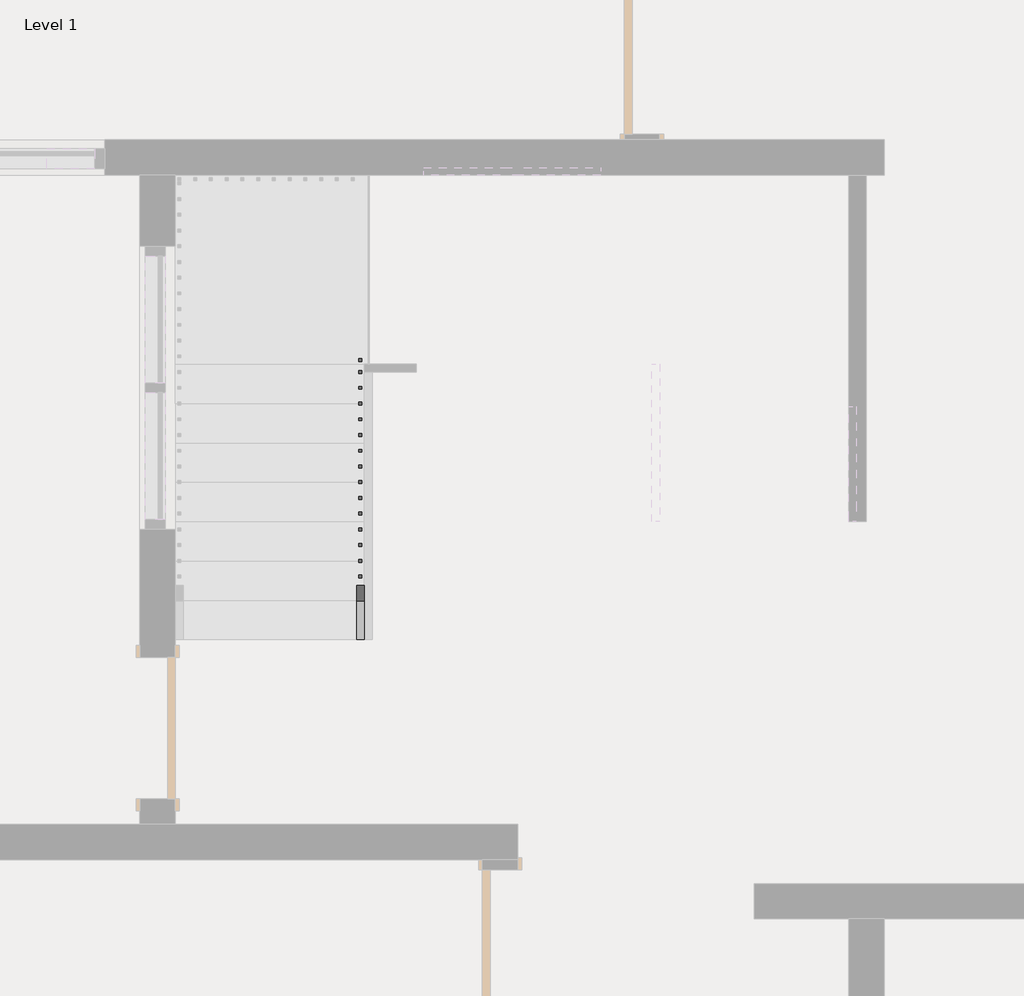
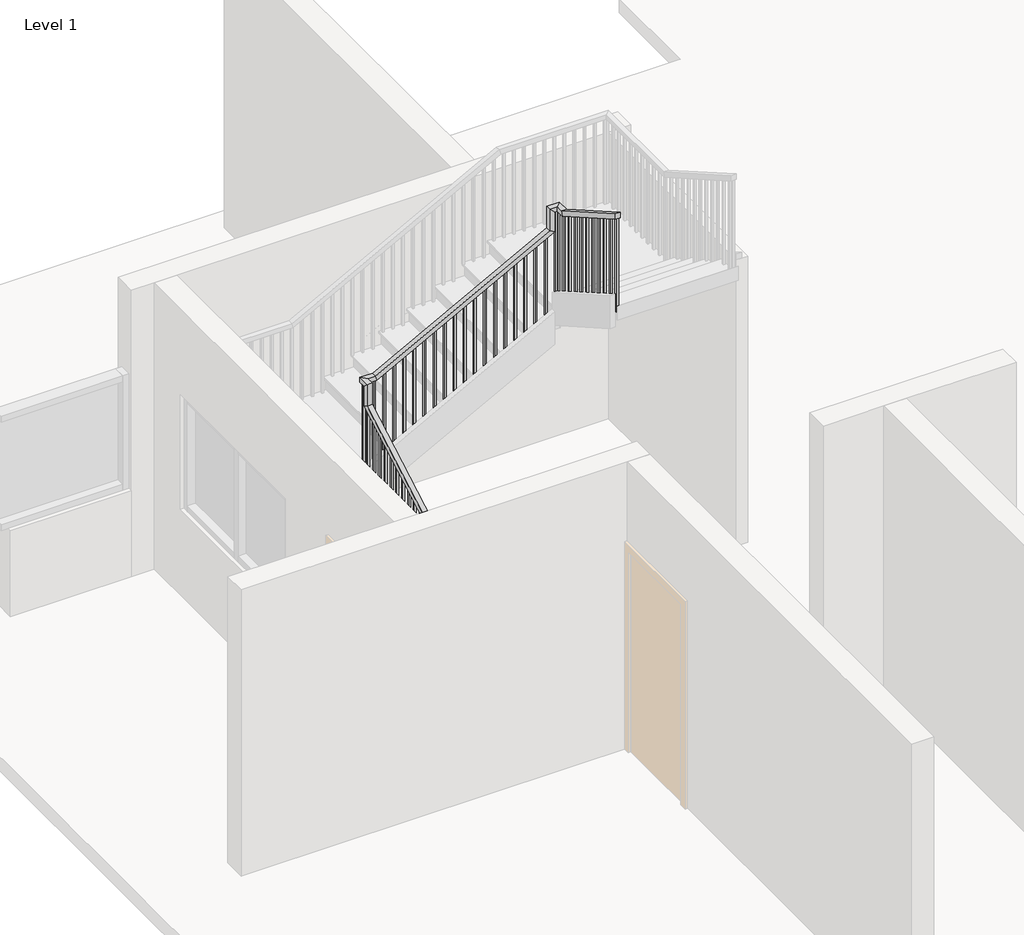
# One storey, part 8 of 9: 1 railing.
"""IFC4 building model written with IfcOpenShell, lengths in millimetres."""

from ifc_helpers import new_model, si_unit, frame, origin, place, context, project, spatial, polyline, outline, extrude, faceted_brep, element, save

model = new_model("IFC4")

# Units and contexts
model_context = context("Model", 3, world=origin())
ifc_project = project(units=[si_unit("LENGTHUNIT", "METRE", prefix="MILLI")], contexts=[model_context])

# Site, building, storey
site = spatial("IfcSite", under=ifc_project)
building = spatial("IfcBuilding", under=site)
storey = spatial("IfcBuildingStorey", under=building, Name="Level 1", Elevation=0.0)

# Railing
placement = place(None, origin())
element("IfcRailing", 1, ObjectType="Handrail - Rectangular", at=placement, inside=storey, context=model_context, shape_type="SolidModel", body=[
    faceted_brep([(14461.3100959, 14647.8480703, 1059.5428571), (14461.3100959, 14647.8480703, 1001.0339009), (14512.1100959, 14647.8480703, 1001.0339009), (14512.1100959, 14647.8480703, 1059.5428571), (14461.3100959, 16349.6480703, 2032.0), (14461.3100959, 16400.4480703, 2002.5196152), (14512.1100959, 16400.4480703, 2002.5196152), (14512.1100959, 16349.6480703, 2032.0), (14461.3100959, 16349.6480703, 2261.3257143), (14461.3100959, 16400.4480703, 2210.5257143), (14512.1100959, 16400.4480703, 2210.5257143), (14512.1100959, 16349.6480703, 2261.3257143), (14461.3100959, 16476.6480703, 2261.3257143), (14461.3100959, 16476.6480703, 2210.5257143), (14512.1100959, 16425.8480703, 2210.5257143), (14512.1100959, 16425.8480703, 2261.3257143), (14588.3100959, 16476.6480703, 2261.3257143), (14601.0100959, 16476.6480703, 2210.5257143), (14601.0100959, 16425.8480703, 2210.5257143), (14588.3100959, 16425.8480703, 2261.3257143), (16340.9100959, 16476.6480703, 3196.0457143), (16391.7100959, 16476.6480703, 3165.5657143), (16391.7100959, 16425.8480703, 3165.5657143), (16340.9100959, 16425.8480703, 3196.0457143), (16340.9100959, 16476.6480703, 3425.3714286), (16391.7100959, 16476.6480703, 3374.5714286), (16391.7100959, 16425.8480703, 3374.5714286), (16340.9100959, 16425.8480703, 3425.3714286), (16467.9100959, 16476.6480703, 3425.3714286), (16467.9100959, 16476.6480703, 3374.5714286), (16417.1100959, 16425.8480703, 3374.5714286), (16417.1100959, 16425.8480703, 3425.3714286), (16467.9100959, 16349.6480703, 3425.3714286), (16467.9100959, 16336.1573969, 3374.5714286), (16417.1100959, 16336.1573969, 3374.5714286), (16417.1100959, 16349.6480703, 3425.3714286), (16467.9100959, 15409.8480703, 3962.4), (16417.1100959, 15409.8480703, 3962.4), (16417.1100959, 15409.8480703, 3903.8910438), (16467.9100959, 15409.8480703, 3903.8910438)], [[[0, 1, 2, 3]], [[1, 0, 4, 5]], [[2, 1, 5, 6]], [[3, 2, 6, 7]], [[0, 3, 7, 4]], [[5, 4, 8, 9]], [[6, 5, 9, 10]], [[7, 6, 10, 11]], [[4, 7, 11, 8]], [[9, 8, 12, 13]], [[10, 9, 13, 14]], [[11, 10, 14, 15]], [[8, 11, 15, 12]], [[13, 12, 16, 17]], [[14, 13, 17, 18]], [[15, 14, 18, 19]], [[12, 15, 19, 16]], [[17, 16, 20, 21]], [[18, 17, 21, 22]], [[19, 18, 22, 23]], [[16, 19, 23, 20]], [[21, 20, 24, 25]], [[22, 21, 25, 26]], [[23, 22, 26, 27]], [[20, 23, 27, 24]], [[25, 24, 28, 29]], [[26, 25, 29, 30]], [[27, 26, 30, 31]], [[24, 27, 31, 28]], [[29, 28, 32, 33]], [[30, 29, 33, 34]], [[31, 30, 34, 35]], [[28, 31, 35, 32]], [[36, 37, 38, 39]], [[33, 32, 36, 39]], [[34, 33, 39, 38]], [[35, 34, 38, 37]], [[32, 35, 37, 36]]]),
    extrude(outline(polyline([(15425.7230703, 3894.8196152), (15444.7730703, 3883.9339009), (15444.7730703, 2902.8571429), (15425.7230703, 2902.8571429), (15425.7230703, 3894.8196152)])), frame((16432.9850959, 0.0, 0.0), z_axis=(1.0, 0.0, 0.0), x_axis=(0.0, 1.0, 0.0)), (0.0, 0.0, 1.0), 19.05),
    extrude(outline(polyline([(15527.3230703, 3836.7624723), (15546.3730703, 3825.8767581), (15546.3730703, 2902.8571429), (15527.3230703, 2902.8571429), (15527.3230703, 3836.7624723)])), frame((16432.9850959, 0.0, 0.0), z_axis=(1.0, 0.0, 0.0), x_axis=(0.0, 1.0, 0.0)), (0.0, 0.0, 1.0), 19.05),
    extrude(outline(polyline([(15628.9230703, 3778.7053295), (15647.9730703, 3767.8196152), (15647.9730703, 2902.8571429), (15628.9230703, 2902.8571429), (15628.9230703, 3778.7053295)])), frame((16432.9850959, 0.0, 0.0), z_axis=(1.0, 0.0, 0.0), x_axis=(0.0, 1.0, 0.0)), (0.0, 0.0, 1.0), 19.05),
    extrude(outline(polyline([(15730.5230703, 3720.6481866), (15749.5730703, 3709.7624723), (15749.5730703, 2757.7142857), (15730.5230703, 2757.7142857), (15730.5230703, 3720.6481866)])), frame((16432.9850959, 0.0, 0.0), z_axis=(1.0, 0.0, 0.0), x_axis=(0.0, 1.0, 0.0)), (0.0, 0.0, 1.0), 19.05),
    extrude(outline(polyline([(15832.1230703, 3662.5910438), (15851.1730703, 3651.7053295), (15851.1730703, 2757.7142857), (15832.1230703, 2757.7142857), (15832.1230703, 3662.5910438)])), frame((16432.9850959, 0.0, 0.0), z_axis=(1.0, 0.0, 0.0), x_axis=(0.0, 1.0, 0.0)), (0.0, 0.0, 1.0), 19.05),
    extrude(outline(polyline([(15933.7230703, 3604.5339009), (15952.7730703, 3593.6481866), (15952.7730703, 2612.5714286), (15933.7230703, 2612.5714286), (15933.7230703, 3604.5339009)])), frame((16432.9850959, 0.0, 0.0), z_axis=(1.0, 0.0, 0.0), x_axis=(0.0, 1.0, 0.0)), (0.0, 0.0, 1.0), 19.05),
    extrude(outline(polyline([(16035.3230703, 3546.4767581), (16054.3730703, 3535.5910438), (16054.3730703, 2612.5714286), (16035.3230703, 2612.5714286), (16035.3230703, 3546.4767581)])), frame((16432.9850959, 0.0, 0.0), z_axis=(1.0, 0.0, 0.0), x_axis=(0.0, 1.0, 0.0)), (0.0, 0.0, 1.0), 19.05),
    extrude(outline(polyline([(16136.9230703, 3488.4196152), (16155.9730703, 3477.5339009), (16155.9730703, 2612.5714286), (16136.9230703, 2612.5714286), (16136.9230703, 3488.4196152)])), frame((16432.9850959, 0.0, 0.0), z_axis=(1.0, 0.0, 0.0), x_axis=(0.0, 1.0, 0.0)), (0.0, 0.0, 1.0), 19.05),
    extrude(outline(polyline([(16238.5230703, 3430.3624723), (16257.5730703, 3419.4767581), (16257.5730703, 2467.4285714), (16238.5230703, 2467.4285714), (16238.5230703, 3430.3624723)])), frame((16432.9850959, 0.0, 0.0), z_axis=(1.0, 0.0, 0.0), x_axis=(0.0, 1.0, 0.0)), (0.0, 0.0, 1.0), 19.05),
    extrude(outline(polyline([(16340.1230703, 3372.3053295), (16359.1730703, 3361.4196152), (16359.1730703, 2467.4285714), (16340.1230703, 2467.4285714), (16340.1230703, 3372.3053295)])), frame((16432.9850959, 0.0, 0.0), z_axis=(1.0, 0.0, 0.0), x_axis=(0.0, 1.0, 0.0)), (0.0, 0.0, 1.0), 19.05),
    extrude(outline(polyline([(16407.5850959, 16441.7230703), (16407.5850959, 16460.7730703), (16426.6350959, 16460.7730703), (16426.6350959, 16441.7230703), (16407.5850959, 16441.7230703)])), frame((0.0, 0.0, 2322.2857143), z_axis=(0.0, 0.0, 1.0), x_axis=(1.0, 0.0, 0.0)), (0.0, 0.0, 1.0), 1052.2857143),
    extrude(outline(polyline([(3130.0057143, 16325.0350959), (3119.8457143, 16305.9850959), (2177.1428571, 16305.9850959), (2177.1428571, 16325.0350959), (3130.0057143, 16325.0350959)])), frame((0.0, 16441.7230703, 0.0), z_axis=(0.0, 1.0, 0.0), x_axis=(0.0, 0.0, 1.0)), (0.0, 0.0, 1.0), 19.05),
    extrude(outline(polyline([(3075.8190476, 16223.4350959), (3065.6590476, 16204.3850959), (2177.1428571, 16204.3850959), (2177.1428571, 16223.4350959), (3075.8190476, 16223.4350959)])), frame((0.0, 16441.7230703, 0.0), z_axis=(0.0, 1.0, 0.0), x_axis=(0.0, 0.0, 1.0)), (0.0, 0.0, 1.0), 19.05),
    extrude(outline(polyline([(3021.632381, 16121.8350959), (3011.472381, 16102.7850959), (2032.0, 16102.7850959), (2032.0, 16121.8350959), (3021.632381, 16121.8350959)])), frame((0.0, 16441.7230703, 0.0), z_axis=(0.0, 1.0, 0.0), x_axis=(0.0, 0.0, 1.0)), (0.0, 0.0, 1.0), 19.05),
    extrude(outline(polyline([(2967.4457143, 16020.2350959), (2957.2857143, 16001.1850959), (2032.0, 16001.1850959), (2032.0, 16020.2350959), (2967.4457143, 16020.2350959)])), frame((0.0, 16441.7230703, 0.0), z_axis=(0.0, 1.0, 0.0), x_axis=(0.0, 0.0, 1.0)), (0.0, 0.0, 1.0), 19.05),
    extrude(outline(polyline([(2913.2590476, 15918.6350959), (2903.0990476, 15899.5850959), (2032.0, 15899.5850959), (2032.0, 15918.6350959), (2913.2590476, 15918.6350959)])), frame((0.0, 16441.7230703, 0.0), z_axis=(0.0, 1.0, 0.0), x_axis=(0.0, 0.0, 1.0)), (0.0, 0.0, 1.0), 19.05),
    extrude(outline(polyline([(2859.072381, 15817.0350959), (2848.912381, 15797.9850959), (1886.8571429, 15797.9850959), (1886.8571429, 15817.0350959), (2859.072381, 15817.0350959)])), frame((0.0, 16441.7230703, 0.0), z_axis=(0.0, 1.0, 0.0), x_axis=(0.0, 0.0, 1.0)), (0.0, 0.0, 1.0), 19.05),
    extrude(outline(polyline([(2804.8857143, 15715.4350959), (2794.7257143, 15696.3850959), (1886.8571429, 15696.3850959), (1886.8571429, 15715.4350959), (2804.8857143, 15715.4350959)])), frame((0.0, 16441.7230703, 0.0), z_axis=(0.0, 1.0, 0.0), x_axis=(0.0, 0.0, 1.0)), (0.0, 0.0, 1.0), 19.05),
    extrude(outline(polyline([(2750.6990476, 15613.8350959), (2740.5390476, 15594.7850959), (1886.8571429, 15594.7850959), (1886.8571429, 15613.8350959), (2750.6990476, 15613.8350959)])), frame((0.0, 16441.7230703, 0.0), z_axis=(0.0, 1.0, 0.0), x_axis=(0.0, 0.0, 1.0)), (0.0, 0.0, 1.0), 19.05),
    extrude(outline(polyline([(2696.512381, 15512.2350959), (2686.352381, 15493.1850959), (1741.7142857, 15493.1850959), (1741.7142857, 15512.2350959), (2696.512381, 15512.2350959)])), frame((0.0, 16441.7230703, 0.0), z_axis=(0.0, 1.0, 0.0), x_axis=(0.0, 0.0, 1.0)), (0.0, 0.0, 1.0), 19.05),
    extrude(outline(polyline([(2642.3257143, 15410.6350959), (2632.1657143, 15391.5850959), (1741.7142857, 15391.5850959), (1741.7142857, 15410.6350959), (2642.3257143, 15410.6350959)])), frame((0.0, 16441.7230703, 0.0), z_axis=(0.0, 1.0, 0.0), x_axis=(0.0, 0.0, 1.0)), (0.0, 0.0, 1.0), 19.05),
    extrude(outline(polyline([(2588.1390476, 15309.0350959), (2577.9790476, 15289.9850959), (1596.5714286, 15289.9850959), (1596.5714286, 15309.0350959), (2588.1390476, 15309.0350959)])), frame((0.0, 16441.7230703, 0.0), z_axis=(0.0, 1.0, 0.0), x_axis=(0.0, 0.0, 1.0)), (0.0, 0.0, 1.0), 19.05),
    extrude(outline(polyline([(2533.952381, 15207.4350959), (2523.792381, 15188.3850959), (1596.5714286, 15188.3850959), (1596.5714286, 15207.4350959), (2533.952381, 15207.4350959)])), frame((0.0, 16441.7230703, 0.0), z_axis=(0.0, 1.0, 0.0), x_axis=(0.0, 0.0, 1.0)), (0.0, 0.0, 1.0), 19.05),
    extrude(outline(polyline([(2479.7657143, 15105.8350959), (2469.6057143, 15086.7850959), (1596.5714286, 15086.7850959), (1596.5714286, 15105.8350959), (2479.7657143, 15105.8350959)])), frame((0.0, 16441.7230703, 0.0), z_axis=(0.0, 1.0, 0.0), x_axis=(0.0, 0.0, 1.0)), (0.0, 0.0, 1.0), 19.05),
    extrude(outline(polyline([(2425.5790476, 15004.2350959), (2415.4190476, 14985.1850959), (1451.4285714, 14985.1850959), (1451.4285714, 15004.2350959), (2425.5790476, 15004.2350959)])), frame((0.0, 16441.7230703, 0.0), z_axis=(0.0, 1.0, 0.0), x_axis=(0.0, 0.0, 1.0)), (0.0, 0.0, 1.0), 19.05),
    extrude(outline(polyline([(2371.392381, 14902.6350959), (2361.232381, 14883.5850959), (1451.4285714, 14883.5850959), (1451.4285714, 14902.6350959), (2371.392381, 14902.6350959)])), frame((0.0, 16441.7230703, 0.0), z_axis=(0.0, 1.0, 0.0), x_axis=(0.0, 0.0, 1.0)), (0.0, 0.0, 1.0), 19.05),
    extrude(outline(polyline([(2317.2057143, 14801.0350959), (2307.0457143, 14781.9850959), (1451.4285714, 14781.9850959), (1451.4285714, 14801.0350959), (2317.2057143, 14801.0350959)])), frame((0.0, 16441.7230703, 0.0), z_axis=(0.0, 1.0, 0.0), x_axis=(0.0, 0.0, 1.0)), (0.0, 0.0, 1.0), 19.05),
    extrude(outline(polyline([(2263.0190476, 14699.4350959), (2252.8590476, 14680.3850959), (1306.2857143, 14680.3850959), (1306.2857143, 14699.4350959), (2263.0190476, 14699.4350959)])), frame((0.0, 16441.7230703, 0.0), z_axis=(0.0, 1.0, 0.0), x_axis=(0.0, 0.0, 1.0)), (0.0, 0.0, 1.0), 19.05),
    extrude(outline(polyline([(2208.832381, 14597.8350959), (2198.672381, 14578.7850959), (1306.2857143, 14578.7850959), (1306.2857143, 14597.8350959), (2208.832381, 14597.8350959)])), frame((0.0, 16441.7230703, 0.0), z_axis=(0.0, 1.0, 0.0), x_axis=(0.0, 0.0, 1.0)), (0.0, 0.0, 1.0), 19.05),
    extrude(outline(polyline([(14496.2350959, 16365.5230703), (14477.1850959, 16365.5230703), (14477.1850959, 16384.5730703), (14496.2350959, 16384.5730703), (14496.2350959, 16365.5230703)])), frame((0.0, 0.0, 1016.0), z_axis=(0.0, 0.0, 1.0), x_axis=(1.0, 0.0, 0.0)), (0.0, 0.0, 1.0), 1194.5257143),
    extrude(outline(polyline([(16263.9230703, 1924.5053295), (16282.9730703, 1935.3910438), (16282.9730703, 1016.0), (16263.9230703, 1016.0), (16263.9230703, 1924.5053295)])), frame((14477.1850959, 0.0, 0.0), z_axis=(1.0, 0.0, 0.0), x_axis=(0.0, 1.0, 0.0)), (0.0, 0.0, 1.0), 19.05),
    extrude(outline(polyline([(16162.3230703, 1866.4481866), (16181.3730703, 1877.3339009), (16181.3730703, 1016.0), (16162.3230703, 1016.0), (16162.3230703, 1866.4481866)])), frame((14477.1850959, 0.0, 0.0), z_axis=(1.0, 0.0, 0.0), x_axis=(0.0, 1.0, 0.0)), (0.0, 0.0, 1.0), 19.05),
    extrude(outline(polyline([(16060.7230703, 1808.3910438), (16079.7730703, 1819.2767581), (16079.7730703, 870.8571429), (16060.7230703, 870.8571429), (16060.7230703, 1808.3910438)])), frame((14477.1850959, 0.0, 0.0), z_axis=(1.0, 0.0, 0.0), x_axis=(0.0, 1.0, 0.0)), (0.0, 0.0, 1.0), 19.05),
    extrude(outline(polyline([(15959.1230703, 1750.3339009), (15978.1730703, 1761.2196152), (15978.1730703, 870.8571429), (15959.1230703, 870.8571429), (15959.1230703, 1750.3339009)])), frame((14477.1850959, 0.0, 0.0), z_axis=(1.0, 0.0, 0.0), x_axis=(0.0, 1.0, 0.0)), (0.0, 0.0, 1.0), 19.05),
    extrude(outline(polyline([(15857.5230703, 1692.2767581), (15876.5730703, 1703.1624723), (15876.5730703, 725.7142857), (15857.5230703, 725.7142857), (15857.5230703, 1692.2767581)])), frame((14477.1850959, 0.0, 0.0), z_axis=(1.0, 0.0, 0.0), x_axis=(0.0, 1.0, 0.0)), (0.0, 0.0, 1.0), 19.05),
    extrude(outline(polyline([(15755.9230703, 1634.2196152), (15774.9730703, 1645.1053295), (15774.9730703, 725.7142857), (15755.9230703, 725.7142857), (15755.9230703, 1634.2196152)])), frame((14477.1850959, 0.0, 0.0), z_axis=(1.0, 0.0, 0.0), x_axis=(0.0, 1.0, 0.0)), (0.0, 0.0, 1.0), 19.05),
    extrude(outline(polyline([(15654.3230703, 1576.1624723), (15673.3730703, 1587.0481866), (15673.3730703, 725.7142857), (15654.3230703, 725.7142857), (15654.3230703, 1576.1624723)])), frame((14477.1850959, 0.0, 0.0), z_axis=(1.0, 0.0, 0.0), x_axis=(0.0, 1.0, 0.0)), (0.0, 0.0, 1.0), 19.05),
    extrude(outline(polyline([(15552.7230703, 1518.1053295), (15571.7730703, 1528.9910438), (15571.7730703, 580.5714286), (15552.7230703, 580.5714286), (15552.7230703, 1518.1053295)])), frame((14477.1850959, 0.0, 0.0), z_axis=(1.0, 0.0, 0.0), x_axis=(0.0, 1.0, 0.0)), (0.0, 0.0, 1.0), 19.05),
    extrude(outline(polyline([(15451.1230703, 1460.0481866), (15470.1730703, 1470.9339009), (15470.1730703, 580.5714286), (15451.1230703, 580.5714286), (15451.1230703, 1460.0481866)])), frame((14477.1850959, 0.0, 0.0), z_axis=(1.0, 0.0, 0.0), x_axis=(0.0, 1.0, 0.0)), (0.0, 0.0, 1.0), 19.05),
    extrude(outline(polyline([(15349.5230703, 1401.9910438), (15368.5730703, 1412.8767581), (15368.5730703, 435.4285714), (15349.5230703, 435.4285714), (15349.5230703, 1401.9910438)])), frame((14477.1850959, 0.0, 0.0), z_axis=(1.0, 0.0, 0.0), x_axis=(0.0, 1.0, 0.0)), (0.0, 0.0, 1.0), 19.05),
    extrude(outline(polyline([(15247.9230703, 1343.9339009), (15266.9730703, 1354.8196152), (15266.9730703, 435.4285714), (15247.9230703, 435.4285714), (15247.9230703, 1343.9339009)])), frame((14477.1850959, 0.0, 0.0), z_axis=(1.0, 0.0, 0.0), x_axis=(0.0, 1.0, 0.0)), (0.0, 0.0, 1.0), 19.05),
    extrude(outline(polyline([(15146.3230703, 1285.8767581), (15165.3730703, 1296.7624723), (15165.3730703, 435.4285714), (15146.3230703, 435.4285714), (15146.3230703, 1285.8767581)])), frame((14477.1850959, 0.0, 0.0), z_axis=(1.0, 0.0, 0.0), x_axis=(0.0, 1.0, 0.0)), (0.0, 0.0, 1.0), 19.05),
    extrude(outline(polyline([(15044.7230703, 1227.8196152), (15063.7730703, 1238.7053295), (15063.7730703, 290.2857143), (15044.7230703, 290.2857143), (15044.7230703, 1227.8196152)])), frame((14477.1850959, 0.0, 0.0), z_axis=(1.0, 0.0, 0.0), x_axis=(0.0, 1.0, 0.0)), (0.0, 0.0, 1.0), 19.05),
    extrude(outline(polyline([(14943.1230703, 1169.7624723), (14962.1730703, 1180.6481866), (14962.1730703, 290.2857143), (14943.1230703, 290.2857143), (14943.1230703, 1169.7624723)])), frame((14477.1850959, 0.0, 0.0), z_axis=(1.0, 0.0, 0.0), x_axis=(0.0, 1.0, 0.0)), (0.0, 0.0, 1.0), 19.05),
    extrude(outline(polyline([(14841.5230703, 1111.7053295), (14860.5730703, 1122.5910438), (14860.5730703, 145.1428571), (14841.5230703, 145.1428571), (14841.5230703, 1111.7053295)])), frame((14477.1850959, 0.0, 0.0), z_axis=(1.0, 0.0, 0.0), x_axis=(0.0, 1.0, 0.0)), (0.0, 0.0, 1.0), 19.05),
    extrude(outline(polyline([(14739.9230703, 1053.6481866), (14758.9730703, 1064.5339009), (14758.9730703, 145.1428571), (14739.9230703, 145.1428571), (14739.9230703, 1053.6481866)])), frame((14477.1850959, 0.0, 0.0), z_axis=(1.0, 0.0, 0.0), x_axis=(0.0, 1.0, 0.0)), (0.0, 0.0, 1.0), 19.05),
    extrude(outline(polyline([(16432.9850959, 16441.7230703), (16432.9850959, 16460.7730703), (16452.0350959, 16460.7730703), (16452.0350959, 16441.7230703), (16432.9850959, 16441.7230703)])), frame((0.0, 0.0, 2322.2857143), z_axis=(0.0, 0.0, 1.0), x_axis=(1.0, 0.0, 0.0)), (0.0, 0.0, 1.0), 1052.2857143),
    extrude(outline(polyline([(14496.2350959, 16441.7230703), (14477.1850959, 16441.7230703), (14477.1850959, 16460.7730703), (14496.2350959, 16460.7730703), (14496.2350959, 16441.7230703)])), frame((0.0, 0.0, 1161.1428571), z_axis=(0.0, 0.0, 1.0), x_axis=(1.0, 0.0, 0.0)), (0.0, 0.0, 1.0), 1049.3828571),
    extrude(outline(polyline([(15409.8480703, 3903.8910438), (15428.8980703, 3893.0053295), (15428.8980703, 2902.8571429), (15409.8480703, 2902.8571429), (15409.8480703, 3903.8910438)])), frame((16432.9850959, 0.0, 0.0), z_axis=(1.0, 0.0, 0.0), x_axis=(0.0, 1.0, 0.0)), (0.0, 0.0, 1.0), 19.05),
    extrude(outline(polyline([(14647.8480703, 1001.0339009), (14666.8980703, 1011.9196152), (14666.8980703, 145.1428571), (14647.8480703, 145.1428571), (14647.8480703, 1001.0339009)])), frame((14477.1850959, 0.0, 0.0), z_axis=(1.0, 0.0, 0.0), x_axis=(0.0, 1.0, 0.0)), (0.0, 0.0, 1.0), 19.05),
])

save(model, "model.ifc")

# Revit data of these elements
# Type "Handrail - Rectangular"
#   Assembly Code = "C2010400"
#   built-in parameter 1008612 = 0.0416667 (stored number, unit not read)
#   built-in parameter 1008611 = 0.0416667 (stored number, unit not read)
#   built-in parameter 1008609 = 0.333333 (stored number, unit not read)
#   built-in parameter 1008604 = 0.166667 (stored number, unit not read)
#   built-in parameter 1008603 = 0.166667 (stored number, unit not read)
#   Railing Height = 3' - 0"
#   built-in parameter 1008630 = 2
#   built-in parameter 1008610 = 2
#   built-in parameter 1008618 = Baluster - Square : 3/4"
# Element 1 (IfcRailing, "Handrail - Rectangular")
#   Phase Created = New Construction
